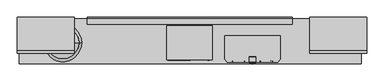
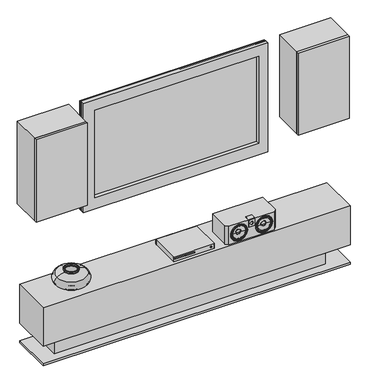
"""IFC4 building model written with IfcOpenShell, lengths in millimetres: furniture geometry."""

from ifc_helpers import new_model, si_unit, point, frame, frame_2d, origin, place, context, project, spatial, polyline, circle_curve, ellipse_curve, trimmed, segment, composite_curve, outline, extrude, source, transform, mapped, element, save
from ifc_brep_helpers import plane_surface, cylinder_surface, revolved_surface, advanced_brep


def furniture_82e6548d(model_context):
    return source(origin(), model_context, "Body", "SolidModel", [
        advanced_brep(
        [(-639.7449376, -196.5814234, 623.1824519), (-549.7449376, -196.5814234, 623.1824519), (-552.6293304, -196.5814234, 620.2980592), (-636.8605449, -196.5814234, 620.2980592), (-639.7449376, -196.5814234, 624.4168309), (-549.7449376, -196.5814234, 624.4168309), (-642.5429469, -196.5814234, 628.1680622), (-546.9469284, -196.5814234, 628.1680622), (-732.6689597, -196.5814234, 648.0450381), (-456.8209156, -196.5814234, 648.0450381), (-737.117516, -196.5814234, 732.9285485), (-452.3723593, -196.5814234, 732.9285485), (-662.9428076, -196.5814234, 762.897076), (-526.5470677, -196.5814234, 762.897076), (-655.9949338, -196.5814234, 766.1369227), (-533.4949414, -196.5814234, 766.1369227), (-660.6249856, -196.5814234, 773.2665773), (-528.8648897, -196.5814234, 773.2665773), (-660.6249856, -196.5814234, 780.1412568), (-528.8648897, -196.5814234, 780.1412568), (-652.9929948, -196.5814234, 780.1412568), (-536.4968805, -196.5814234, 780.1412568), (-649.5413299, -196.5814234, 775.2117685), (-539.9485454, -196.5814234, 775.2117685), (-651.8181703, -196.5814234, 761.8066565), (-537.671705, -196.5814234, 761.8066565), (-661.7982324, -196.5814234, 757.0072587), (-527.6916429, -196.5814234, 757.0072587), (-733.8494437, -196.5814234, 727.8966798), (-455.6404316, -196.5814234, 727.8966798), (-729.9447637, -196.5814234, 653.3909483), (-459.5451115, -196.5814234, 653.3909483), (-639.3868915, -196.5814234, 634.3217368), (-550.1029838, -196.5814234, 634.3217368), (-632.2712578, -196.5814234, 629.6724919), (-557.2186175, -196.5814234, 629.6724919), (-626.4265689, -196.5814234, 626.2980592), (-563.0633064, -196.5814234, 626.2980592), (-594.7449376, -196.5814234, 626.2980592), (-594.7449376, -196.5814234, 620.2980592)],
        [
            (0, 1, circle_curve(frame((-594.7449376, -196.5814234, 623.1824519), z_axis=(0.0, 0.0, -1.0), x_axis=(1.0, 0.0, 0.0)), 45.0)),
            (1, 2, circle_curve(frame((-552.6293304, -196.5814234, 623.1824519), z_axis=(0.0, 1.0, 0.0), x_axis=(1.0, 0.0, 0.0)), 2.8843927)),
            (2, 3, circle_curve(frame((-594.7449376, -196.5814234, 620.2980592), z_axis=(0.0, 0.0, 1.0), x_axis=(1.0, 0.0, 0.0)), 42.1156073)),
            (3, 0, circle_curve(frame((-636.8605449, -196.5814234, 623.1824519), z_axis=(0.0, 1.0, 0.0), x_axis=(-1.0, 0.0, 0.0)), 2.8843927)),
            (1, 0, circle_curve(frame((-594.7449376, -196.5814234, 623.1824519), z_axis=(0.0, 0.0, -1.0), x_axis=(1.0, 0.0, 0.0)), 45.0)),
            (3, 2, circle_curve(frame((-594.7449376, -196.5814234, 620.2980592), z_axis=(0.0, 0.0, 1.0), x_axis=(1.0, 0.0, 0.0)), 42.1156073)),
            (4, 5, circle_curve(frame((-594.7449376, -196.5814234, 624.4168309), z_axis=(0.0, 0.0, -1.0), x_axis=(1.0, 0.0, 0.0)), 45.0)),
            (5, 1),
            (0, 4),
            (5, 4, circle_curve(frame((-594.7449376, -196.5814234, 624.4168309), z_axis=(0.0, 0.0, -1.0), x_axis=(1.0, 0.0, 0.0)), 45.0)),
            (6, 7, circle_curve(frame((-594.7449376, -196.5814234, 628.1680622), z_axis=(0.0, 0.0, -1.0), x_axis=(1.0, 0.0, 0.0)), 47.7980093)),
            (7, 5, circle_curve(frame((-545.7501654, -196.5814234, 624.3562871), z_axis=(0.0, -1.0, 0.0), x_axis=(1.0, 0.0, 0.0)), 3.995231)),
            (4, 6, circle_curve(frame((-643.7397099, -196.5814234, 624.3562871), z_axis=(0.0, -1.0, 0.0), x_axis=(-1.0, 0.0, 0.0)), 3.995231)),
            (7, 6, circle_curve(frame((-594.7449376, -196.5814234, 628.1680622), z_axis=(0.0, 0.0, -1.0), x_axis=(1.0, 0.0, 0.0)), 47.7980093)),
            (8, 9, circle_curve(frame((-594.7449376, -196.5814234, 648.0450381), z_axis=(0.0, 0.0, -1.0), x_axis=(1.0, 0.0, 0.0)), 137.9240221)),
            (9, 7, circle_curve(frame((-540.1329588, -196.5814234, 811.5350037), z_axis=(0.0, 1.0, 0.0), x_axis=(1.0, 0.0, 0.0)), 183.4935024)),
            (6, 8, circle_curve(frame((-649.3569165, -196.5814234, 811.5350037), z_axis=(0.0, 1.0, 0.0), x_axis=(-1.0, 0.0, 0.0)), 183.4935024)),
            (9, 8, circle_curve(frame((-594.7449376, -196.5814234, 648.0450381), z_axis=(0.0, 0.0, -1.0), x_axis=(1.0, 0.0, 0.0)), 137.9240221)),
            (10, 11, circle_curve(frame((-594.7449376, -196.5814234, 732.9285485), z_axis=(0.0, 0.0, -1.0), x_axis=(1.0, 0.0, 0.0)), 142.3725784)),
            (11, 9, circle_curve(frame((-479.1030741, -196.5814234, 691.7711212), z_axis=(0.0, 1.0, 0.0), x_axis=(1.0, 0.0, 0.0)), 49.0761137)),
            (8, 10, circle_curve(frame((-710.3868012, -196.5814234, 691.7711212), z_axis=(0.0, 1.0, 0.0), x_axis=(-1.0, 0.0, 0.0)), 49.0761137)),
            (11, 10, circle_curve(frame((-594.7449376, -196.5814234, 732.9285485), z_axis=(0.0, 0.0, -1.0), x_axis=(1.0, 0.0, 0.0)), 142.3725784)),
            (12, 13, circle_curve(frame((-594.7449376, -196.5814234, 762.897076), z_axis=(0.0, 0.0, -1.0), x_axis=(1.0, 0.0, 0.0)), 68.19787)),
            (13, 11, circle_curve(frame((-566.5275973, -196.5814234, 557.1631061), z_axis=(0.0, 1.0, 0.0), x_axis=(1.0, 0.0, 0.0)), 209.5827023)),
            (10, 12, circle_curve(frame((-622.962278, -196.5814234, 557.1631061), z_axis=(0.0, 1.0, 0.0), x_axis=(-1.0, 0.0, 0.0)), 209.5827023)),
            (13, 12, circle_curve(frame((-594.7449376, -196.5814234, 762.897076), z_axis=(0.0, 0.0, -1.0), x_axis=(1.0, 0.0, 0.0)), 68.19787)),
            (14, 15, circle_curve(frame((-594.7449376, -196.5814234, 766.1369227), z_axis=(0.0, 0.0, -1.0), x_axis=(1.0, 0.0, 0.0)), 61.2499962)),
            (15, 13, circle_curve(frame((-523.5251563, -196.5814234, 778.447391), z_axis=(0.0, -1.0, 0.0), x_axis=(1.0, 0.0, 0.0)), 15.8412198)),
            (12, 14, circle_curve(frame((-665.964719, -196.5814234, 778.447391), z_axis=(0.0, -1.0, 0.0), x_axis=(-1.0, 0.0, 0.0)), 15.8412198)),
            (15, 14, circle_curve(frame((-594.7449376, -196.5814234, 766.1369227), z_axis=(0.0, 0.0, -1.0), x_axis=(1.0, 0.0, 0.0)), 61.2499962)),
            (16, 17, circle_curve(frame((-594.7449376, -196.5814234, 773.2665773), z_axis=(0.0, 0.0, -1.0), x_axis=(1.0, 0.0, 0.0)), 65.880048)),
            (17, 15, circle_curve(frame((-530.8050666, -196.5814234, 769.4583202), z_axis=(0.0, -1.0, 0.0), x_axis=(1.0, 0.0, 0.0)), 4.2740038)),
            (14, 16, circle_curve(frame((-658.6848087, -196.5814234, 769.4583202), z_axis=(0.0, -1.0, 0.0), x_axis=(-1.0, 0.0, 0.0)), 4.2740038)),
            (17, 16, circle_curve(frame((-594.7449376, -196.5814234, 773.2665773), z_axis=(0.0, 0.0, -1.0), x_axis=(1.0, 0.0, 0.0)), 65.880048)),
            (18, 19, circle_curve(frame((-594.7449376, -196.5814234, 780.1412568), z_axis=(0.0, 0.0, -1.0), x_axis=(1.0, 0.0, 0.0)), 65.880048)),
            (19, 17, circle_curve(frame((-528.8648897, -196.5814234, 776.703917), z_axis=(0.0, 1.0, 0.0), x_axis=(1.0, 0.0, 0.0)), 3.4373398)),
            (16, 18, circle_curve(frame((-660.6249856, -196.5814234, 776.703917), z_axis=(0.0, 1.0, 0.0), x_axis=(-1.0, 0.0, 0.0)), 3.4373398)),
            (19, 18, circle_curve(frame((-594.7449376, -196.5814234, 780.1412568), z_axis=(0.0, 0.0, -1.0), x_axis=(1.0, 0.0, 0.0)), 65.880048)),
            (20, 21, circle_curve(frame((-594.7449376, -196.5814234, 780.1412568), z_axis=(0.0, 0.0, -1.0), x_axis=(1.0, 0.0, 0.0)), 58.2480571)),
            (21, 19),
            (18, 20),
            (21, 20, circle_curve(frame((-594.7449376, -196.5814234, 780.1412568), z_axis=(0.0, 0.0, -1.0), x_axis=(1.0, 0.0, 0.0)), 58.2480571)),
            (22, 23, circle_curve(frame((-594.7449376, -196.5814234, 775.2117685), z_axis=(0.0, 0.0, -1.0), x_axis=(1.0, 0.0, 0.0)), 54.7963923)),
            (23, 21, circle_curve(frame((-536.4968805, -196.5814234, 776.4680717), z_axis=(0.0, 1.0, 0.0), x_axis=(1.0, 0.0, 0.0)), 3.673185)),
            (20, 22, circle_curve(frame((-652.9929948, -196.5814234, 776.4680717), z_axis=(0.0, 1.0, 0.0), x_axis=(-1.0, 0.0, 0.0)), 3.673185)),
            (23, 22, circle_curve(frame((-594.7449376, -196.5814234, 775.2117685), z_axis=(0.0, 0.0, -1.0), x_axis=(1.0, 0.0, 0.0)), 54.7963923)),
            (24, 25, circle_curve(frame((-594.7449376, -196.5814234, 761.8066565), z_axis=(0.0, 0.0, -1.0), x_axis=(1.0, 0.0, 0.0)), 57.0732327)),
            (25, 23, circle_curve(frame((-508.2403508, -196.5814234, 773.7014481), z_axis=(0.0, 1.0, 0.0), x_axis=(1.0, 0.0, 0.0)), 31.7441439)),
            (22, 24, circle_curve(frame((-681.2495245, -196.5814234, 773.7014481), z_axis=(0.0, 1.0, 0.0), x_axis=(-1.0, 0.0, 0.0)), 31.7441439)),
            (25, 24, circle_curve(frame((-594.7449376, -196.5814234, 761.8066565), z_axis=(0.0, 0.0, -1.0), x_axis=(1.0, 0.0, 0.0)), 57.0732327)),
            (26, 27, circle_curve(frame((-594.7449376, -196.5814234, 757.0072587), z_axis=(0.0, 0.0, -1.0), x_axis=(1.0, 0.0, 0.0)), 67.0532947)),
            (27, 25, circle_curve(frame((-523.5251563, -196.5814234, 778.447391), z_axis=(0.0, 1.0, 0.0), x_axis=(1.0, 0.0, 0.0)), 21.8412198)),
            (24, 26, circle_curve(frame((-665.964719, -196.5814234, 778.447391), z_axis=(0.0, 1.0, 0.0), x_axis=(-1.0, 0.0, 0.0)), 21.8412198)),
            (27, 26, circle_curve(frame((-594.7449376, -196.5814234, 757.0072587), z_axis=(0.0, 0.0, -1.0), x_axis=(1.0, 0.0, 0.0)), 67.0532947)),
            (28, 29, circle_curve(frame((-594.7449376, -196.5814234, 727.8966798), z_axis=(0.0, 0.0, -1.0), x_axis=(1.0, 0.0, 0.0)), 139.104506)),
            (29, 27, circle_curve(frame((-566.5275973, -196.5814234, 557.1631061), z_axis=(0.0, -1.0, 0.0), x_axis=(1.0, 0.0, 0.0)), 203.5827023)),
            (26, 28, circle_curve(frame((-622.962278, -196.5814234, 557.1631061), z_axis=(0.0, -1.0, 0.0), x_axis=(-1.0, 0.0, 0.0)), 203.5827023)),
            (29, 28, circle_curve(frame((-594.7449376, -196.5814234, 727.8966798), z_axis=(0.0, 0.0, -1.0), x_axis=(1.0, 0.0, 0.0)), 139.104506)),
            (30, 31, circle_curve(frame((-594.7449376, -196.5814234, 653.3909483), z_axis=(0.0, 0.0, -1.0), x_axis=(1.0, 0.0, 0.0)), 135.1998261)),
            (31, 29, circle_curve(frame((-479.1030741, -196.5814234, 691.7711212), z_axis=(0.0, -1.0, 0.0), x_axis=(1.0, 0.0, 0.0)), 43.0761137)),
            (28, 30, circle_curve(frame((-710.3868012, -196.5814234, 691.7711212), z_axis=(0.0, -1.0, 0.0), x_axis=(-1.0, 0.0, 0.0)), 43.0761137)),
            (31, 30, circle_curve(frame((-594.7449376, -196.5814234, 653.3909483), z_axis=(0.0, 0.0, -1.0), x_axis=(1.0, 0.0, 0.0)), 135.1998261)),
            (32, 33, circle_curve(frame((-594.7449376, -196.5814234, 634.3217368), z_axis=(0.0, 0.0, -1.0), x_axis=(1.0, 0.0, 0.0)), 44.6419538)),
            (33, 31, circle_curve(frame((-540.1329588, -196.5814234, 811.5350037), z_axis=(0.0, -1.0, 0.0), x_axis=(1.0, 0.0, 0.0)), 177.4935024)),
            (30, 32, circle_curve(frame((-649.3569165, -196.5814234, 811.5350037), z_axis=(0.0, -1.0, 0.0), x_axis=(-1.0, 0.0, 0.0)), 177.4935024)),
            (33, 32, circle_curve(frame((-594.7449376, -196.5814234, 634.3217368), z_axis=(0.0, 0.0, -1.0), x_axis=(1.0, 0.0, 0.0)), 44.6419538)),
            (34, 35, circle_curve(frame((-594.7449376, -196.5814234, 629.6724919), z_axis=(0.0, 0.0, -1.0), x_axis=(1.0, 0.0, 0.0)), 37.5263202)),
            (35, 33, circle_curve(frame((-549.3684369, -196.5814234, 625.4276845), z_axis=(0.0, 1.0, 0.0), x_axis=(1.0, 0.0, 0.0)), 8.9243333)),
            (32, 34, circle_curve(frame((-640.1214384, -196.5814234, 625.4276845), z_axis=(0.0, 1.0, 0.0), x_axis=(-1.0, 0.0, 0.0)), 8.9243333)),
            (35, 34, circle_curve(frame((-594.7449376, -196.5814234, 629.6724919), z_axis=(0.0, 0.0, -1.0), x_axis=(1.0, 0.0, 0.0)), 37.5263202)),
            (36, 37, circle_curve(frame((-594.7449376, -196.5814234, 626.2980592), z_axis=(0.0, 0.0, -1.0), x_axis=(1.0, 0.0, 0.0)), 31.6816313)),
            (37, 35, circle_curve(frame((-563.1842649, -196.5814234, 633.2564309), z_axis=(0.0, -1.0, 0.0), x_axis=(1.0, 0.0, 0.0)), 6.9594229)),
            (34, 36, circle_curve(frame((-626.3056104, -196.5814234, 633.2564309), z_axis=(0.0, -1.0, 0.0), x_axis=(-1.0, 0.0, 0.0)), 6.9594229)),
            (37, 36, circle_curve(frame((-594.7449376, -196.5814234, 626.2980592), z_axis=(0.0, 0.0, -1.0), x_axis=(1.0, 0.0, 0.0)), 31.6816313)),
            (38, 37),
            (36, 38),
            (2, 39),
            (39, 3),
        ],
        [
            revolved_surface(trimmed(ellipse_curve(frame((-552.6293304, -196.5814234, 623.1824519), z_axis=(0.0, -1.0, 0.0), x_axis=(1.0, 0.0, 0.0)), 2.8843927, 2.8843927), [point((-552.6293304, -196.5814234, 620.2980592))], [point((-549.7449376, -196.5814234, 623.1824519))], True, "CARTESIAN"), (-594.7449376, -196.5814234, 800.1412568), (0.0, 0.0, 1.0)),
            cylinder_surface(frame((-594.7449376, -196.5814234, 800.1412568), z_axis=(0.0, 0.0, 1.0), x_axis=(1.0, 0.0, 0.0)), 45.0),
            revolved_surface(trimmed(ellipse_curve(frame((-545.7501654, -196.5814234, 624.3562871), z_axis=(0.0, 1.0, 0.0), x_axis=(1.0, 0.0, 0.0)), 3.995231, 3.995231), [point((-549.7449376, -196.5814234, 624.4168309))], [point((-546.9469284, -196.5814234, 628.1680622))], True, "CARTESIAN"), (-594.7449376, -196.5814234, 800.1412568), (0.0, 0.0, 1.0)),
            revolved_surface(trimmed(ellipse_curve(frame((-540.1329588, -196.5814234, 811.5350037), z_axis=(0.0, -1.0, 0.0), x_axis=(1.0, 0.0, 0.0)), 183.4935024, 183.4935024), [point((-546.9469284, -196.5814234, 628.1680622))], [point((-456.8209156, -196.5814234, 648.0450381))], True, "CARTESIAN"), (-594.7449376, -196.5814234, 800.1412568), (0.0, 0.0, 1.0)),
            revolved_surface(trimmed(ellipse_curve(frame((-479.1030741, -196.5814234, 691.7711212), z_axis=(0.0, -1.0, 0.0), x_axis=(1.0, 0.0, 0.0)), 49.0761137, 49.0761137), [point((-456.8209156, -196.5814234, 648.0450381))], [point((-452.3723593, -196.5814234, 732.9285485))], True, "CARTESIAN"), (-594.7449376, -196.5814234, 800.1412568), (0.0, 0.0, 1.0)),
            revolved_surface(trimmed(ellipse_curve(frame((-566.5275973, -196.5814234, 557.1631061), z_axis=(0.0, -1.0, 0.0), x_axis=(1.0, 0.0, 0.0)), 209.5827023, 209.5827023), [point((-452.3723593, -196.5814234, 732.9285485))], [point((-526.5470677, -196.5814234, 762.897076))], True, "CARTESIAN"), (-594.7449376, -196.5814234, 800.1412568), (0.0, 0.0, 1.0)),
            revolved_surface(trimmed(ellipse_curve(frame((-523.5251563, -196.5814234, 778.447391), z_axis=(0.0, 1.0, 0.0), x_axis=(1.0, 0.0, 0.0)), 15.8412198, 15.8412198), [point((-526.5470677, -196.5814234, 762.897076))], [point((-533.4949414, -196.5814234, 766.1369227))], True, "CARTESIAN"), (-594.7449376, -196.5814234, 800.1412568), (0.0, 0.0, 1.0)),
            revolved_surface(trimmed(ellipse_curve(frame((-530.8050666, -196.5814234, 769.4583202), z_axis=(0.0, 1.0, 0.0), x_axis=(1.0, 0.0, 0.0)), 4.2740038, 4.2740038), [point((-533.4949414, -196.5814234, 766.1369227))], [point((-528.8648897, -196.5814234, 773.2665773))], True, "CARTESIAN"), (-594.7449376, -196.5814234, 800.1412568), (0.0, 0.0, 1.0)),
            revolved_surface(trimmed(ellipse_curve(frame((-528.8648897, -196.5814234, 776.703917), z_axis=(0.0, -1.0, 0.0), x_axis=(1.0, 0.0, 0.0)), 3.4373398, 3.4373398), [point((-528.8648897, -196.5814234, 773.2665773))], [point((-528.8648897, -196.5814234, 780.1412568))], True, "CARTESIAN"), (-594.7449376, -196.5814234, 800.1412568), (0.0, 0.0, 1.0)),
            plane_surface(frame((-594.7449376, -196.5814234, 780.1412568), z_axis=(0.0, 0.0, 1.0), x_axis=(1.0, 0.0, 0.0))),
            revolved_surface(trimmed(ellipse_curve(frame((-536.4968805, -196.5814234, 776.4680717), z_axis=(0.0, -1.0, 0.0), x_axis=(1.0, 0.0, 0.0)), 3.673185, 3.673185), [point((-536.4968805, -196.5814234, 780.1412568))], [point((-539.9485454, -196.5814234, 775.2117685))], True, "CARTESIAN"), (-594.7449376, -196.5814234, 800.1412568), (0.0, 0.0, 1.0)),
            revolved_surface(trimmed(ellipse_curve(frame((-508.2403508, -196.5814234, 773.7014481), z_axis=(0.0, -1.0, 0.0), x_axis=(1.0, 0.0, 0.0)), 31.7441439, 31.7441439), [point((-539.9485454, -196.5814234, 775.2117685))], [point((-537.671705, -196.5814234, 761.8066565))], True, "CARTESIAN"), (-594.7449376, -196.5814234, 800.1412568), (0.0, 0.0, 1.0)),
            revolved_surface(trimmed(ellipse_curve(frame((-523.5251563, -196.5814234, 778.447391), z_axis=(0.0, -1.0, 0.0), x_axis=(1.0, 0.0, 0.0)), 21.8412198, 21.8412198), [point((-537.671705, -196.5814234, 761.8066565))], [point((-527.6916429, -196.5814234, 757.0072587))], True, "CARTESIAN"), (-594.7449376, -196.5814234, 800.1412568), (0.0, 0.0, 1.0)),
            revolved_surface(trimmed(ellipse_curve(frame((-566.5275973, -196.5814234, 557.1631061), z_axis=(0.0, 1.0, 0.0), x_axis=(1.0, 0.0, 0.0)), 203.5827023, 203.5827023), [point((-527.6916429, -196.5814234, 757.0072587))], [point((-455.6404316, -196.5814234, 727.8966798))], True, "CARTESIAN"), (-594.7449376, -196.5814234, 800.1412568), (0.0, 0.0, 1.0)),
            revolved_surface(trimmed(ellipse_curve(frame((-479.1030741, -196.5814234, 691.7711212), z_axis=(0.0, 1.0, 0.0), x_axis=(1.0, 0.0, 0.0)), 43.0761137, 43.0761137), [point((-455.6404316, -196.5814234, 727.8966798))], [point((-459.5451115, -196.5814234, 653.3909483))], True, "CARTESIAN"), (-594.7449376, -196.5814234, 800.1412568), (0.0, 0.0, 1.0)),
            revolved_surface(trimmed(ellipse_curve(frame((-540.1329588, -196.5814234, 811.5350037), z_axis=(0.0, 1.0, 0.0), x_axis=(1.0, 0.0, 0.0)), 177.4935024, 177.4935024), [point((-459.5451115, -196.5814234, 653.3909483))], [point((-550.1029838, -196.5814234, 634.3217368))], True, "CARTESIAN"), (-594.7449376, -196.5814234, 800.1412568), (0.0, 0.0, 1.0)),
            revolved_surface(trimmed(ellipse_curve(frame((-549.3684369, -196.5814234, 625.4276845), z_axis=(0.0, -1.0, 0.0), x_axis=(1.0, 0.0, 0.0)), 8.9243333, 8.9243333), [point((-550.1029838, -196.5814234, 634.3217368))], [point((-557.2186175, -196.5814234, 629.6724919))], True, "CARTESIAN"), (-594.7449376, -196.5814234, 800.1412568), (0.0, 0.0, 1.0)),
            revolved_surface(trimmed(ellipse_curve(frame((-563.1842649, -196.5814234, 633.2564309), z_axis=(0.0, 1.0, 0.0), x_axis=(1.0, 0.0, 0.0)), 6.9594229, 6.9594229), [point((-557.2186175, -196.5814234, 629.6724919))], [point((-563.0633064, -196.5814234, 626.2980592))], True, "CARTESIAN"), (-594.7449376, -196.5814234, 800.1412568), (0.0, 0.0, 1.0)),
            plane_surface(frame((-594.7449376, -196.5814234, 626.2980592), z_axis=(0.0, 0.0, 1.0), x_axis=(1.0, 0.0, 0.0))),
            plane_surface(frame((-594.7449376, -196.5814234, 620.2980592), z_axis=(0.0, 0.0, -1.0), x_axis=(1.0, 0.0, 0.0))),
        ],
        [
            (0, [[1, 2, 3, 4]]),
            (0, [[5, -4, 6, -2]]),
            (1, [[7, 8, -1, 9]]),
            (1, [[10, -9, -5, -8]]),
            (2, [[11, 12, -7, 13]]),
            (2, [[14, -13, -10, -12]]),
            (3, [[15, 16, -11, 17]]),
            (3, [[18, -17, -14, -16]]),
            (4, [[19, 20, -15, 21]]),
            (4, [[22, -21, -18, -20]]),
            (5, [[23, 24, -19, 25]]),
            (5, [[26, -25, -22, -24]]),
            (6, [[27, 28, -23, 29]]),
            (6, [[30, -29, -26, -28]]),
            (7, [[31, 32, -27, 33]]),
            (7, [[34, -33, -30, -32]]),
            (8, [[35, 36, -31, 37]]),
            (8, [[38, -37, -34, -36]]),
            (9, [[39, 40, -35, 41]]),
            (9, [[42, -41, -38, -40]]),
            (10, [[43, 44, -39, 45]]),
            (10, [[46, -45, -42, -44]]),
            (11, [[47, 48, -43, 49]]),
            (11, [[50, -49, -46, -48]]),
            (12, [[51, 52, -47, 53]]),
            (12, [[54, -53, -50, -52]]),
            (13, [[55, 56, -51, 57]]),
            (13, [[58, -57, -54, -56]]),
            (14, [[59, 60, -55, 61]]),
            (14, [[62, -61, -58, -60]]),
            (15, [[63, 64, -59, 65]]),
            (15, [[66, -65, -62, -64]]),
            (16, [[67, 68, -63, 69]]),
            (16, [[70, -69, -66, -68]]),
            (17, [[71, 72, -67, 73]]),
            (17, [[74, -73, -70, -72]]),
            (18, [[75, -71, 76]]),
            (18, [[-76, -74, -75]]),
            (19, [[-3, 77, 78]]),
            (19, [[-6, -78, -77]]),
        ],
    ),
        advanced_brep(
        [(1262.045258, -367.5, 711.570893), (1119.0326349, -367.5, 711.570893), (1120.5389465, -365.9936884, 711.570893), (1260.5389465, -365.9936884, 711.570893), (1272.0516084, -367.5, 711.570893), (1109.0262846, -367.5, 711.570893), (1273.5389465, -366.0126619, 711.570893), (1107.5389465, -366.0126619, 711.570893), (1273.5389465, -365.0, 711.570893), (1107.5389465, -365.0, 711.570893), (1260.5389465, -365.0, 711.570893), (1120.5389465, -365.0, 711.570893)],
        [
            (0, 1, circle_curve(frame((1190.5389465, -367.5, 711.570893), z_axis=(0.0, -1.0, 0.0), x_axis=(-1.0, 0.0, 0.0)), 71.5063116)),
            (1, 2, circle_curve(frame((1119.0326349, -365.9936884, 711.570893), z_axis=(0.0, 0.0, 1.0), x_axis=(1.0, 0.0, 0.0)), 1.5063116)),
            (2, 3, circle_curve(frame((1190.5389465, -365.9936884, 711.570893), z_axis=(0.0, 1.0, 0.0), x_axis=(-1.0, 0.0, 0.0)), 70.0)),
            (3, 0, circle_curve(frame((1262.045258, -365.9936884, 711.570893), z_axis=(0.0, 0.0, 1.0), x_axis=(-1.0, 0.0, 0.0)), 1.5063116)),
            (1, 0, circle_curve(frame((1190.5389465, -367.5, 711.570893), z_axis=(0.0, -1.0, 0.0), x_axis=(-1.0, 0.0, 0.0)), 71.5063116)),
            (3, 2, circle_curve(frame((1190.5389465, -365.9936884, 711.570893), z_axis=(0.0, 1.0, 0.0), x_axis=(-1.0, 0.0, 0.0)), 70.0)),
            (4, 5, circle_curve(frame((1190.5389465, -367.5, 711.570893), z_axis=(0.0, -1.0, 0.0), x_axis=(-1.0, 0.0, 0.0)), 81.5126619)),
            (5, 1),
            (0, 4),
            (5, 4, circle_curve(frame((1190.5389465, -367.5, 711.570893), z_axis=(0.0, -1.0, 0.0), x_axis=(-1.0, 0.0, 0.0)), 81.5126619)),
            (6, 7, circle_curve(frame((1190.5389465, -366.0126619, 711.570893), z_axis=(0.0, -1.0, 0.0), x_axis=(-1.0, 0.0, 0.0)), 83.0)),
            (7, 5, circle_curve(frame((1109.0262846, -366.0126619, 711.570893), z_axis=(0.0, 0.0, 1.0), x_axis=(1.0, 0.0, 0.0)), 1.4873381)),
            (4, 6, circle_curve(frame((1272.0516084, -366.0126619, 711.570893), z_axis=(0.0, 0.0, 1.0), x_axis=(-1.0, 0.0, 0.0)), 1.4873381)),
            (7, 6, circle_curve(frame((1190.5389465, -366.0126619, 711.570893), z_axis=(0.0, -1.0, 0.0), x_axis=(-1.0, 0.0, 0.0)), 83.0)),
            (8, 9, circle_curve(frame((1190.5389465, -365.0, 711.570893), z_axis=(0.0, -1.0, 0.0), x_axis=(-1.0, 0.0, 0.0)), 83.0)),
            (9, 7),
            (6, 8),
            (9, 8, circle_curve(frame((1190.5389465, -365.0, 711.570893), z_axis=(0.0, -1.0, 0.0), x_axis=(-1.0, 0.0, 0.0)), 83.0)),
            (10, 11, circle_curve(frame((1190.5389465, -365.0, 711.570893), z_axis=(0.0, -1.0, 0.0), x_axis=(-1.0, 0.0, 0.0)), 70.0)),
            (11, 9),
            (8, 10),
            (11, 10, circle_curve(frame((1190.5389465, -365.0, 711.570893), z_axis=(0.0, -1.0, 0.0), x_axis=(-1.0, 0.0, 0.0)), 70.0)),
            (2, 11),
            (10, 3),
        ],
        [
            revolved_surface(trimmed(ellipse_curve(frame((1119.0326349, -365.9936884, 711.570893), z_axis=(0.0, 0.0, -1.0), x_axis=(1.0, 0.0, 0.0)), 1.5063116, 1.5063116), [point((1120.5389465, -365.9936884, 711.570893))], [point((1119.0326349, -367.5, 711.570893))], True, "CARTESIAN"), (1190.5389465, -2974.0581012, 711.570893), (0.0, 1.0, 0.0)),
            plane_surface(frame((1190.5389465, -367.5, 711.570893), z_axis=(0.0, -1.0, 0.0), x_axis=(-1.0, 0.0, 0.0))),
            revolved_surface(trimmed(ellipse_curve(frame((1109.0262846, -366.0126619, 711.570893), z_axis=(0.0, 0.0, -1.0), x_axis=(1.0, 0.0, 0.0)), 1.4873381, 1.4873381), [point((1109.0262846, -367.5, 711.570893))], [point((1107.5389465, -366.0126619, 711.570893))], True, "CARTESIAN"), (1190.5389465, -2974.0581012, 711.570893), (0.0, 1.0, 0.0)),
            cylinder_surface(frame((1190.5389465, -2974.0581012, 711.570893), z_axis=(0.0, 1.0, 0.0), x_axis=(-1.0, 0.0, 0.0)), 83.0),
            plane_surface(frame((1190.5389465, -365.0, 711.570893), z_axis=(0.0, 1.0, 0.0), x_axis=(-1.0, 0.0, 0.0))),
            revolved_surface(polyline([(1120.5389465, -365.0, 711.570893), (1120.5389465, -365.9936883999999, 711.570893)]), (1190.5389465, -2974.0581012, 711.570893), (0.0, 1.0, 0.0)),
        ],
        [
            (0, [[1, 2, 3, 4]]),
            (0, [[5, -4, 6, -2]]),
            (1, [[7, 8, -1, 9]]),
            (1, [[10, -9, -5, -8]]),
            (2, [[11, 12, -7, 13]]),
            (2, [[14, -13, -10, -12]]),
            (3, [[15, 16, -11, 17]]),
            (3, [[18, -17, -14, -16]]),
            (4, [[19, 20, -15, 21]]),
            (4, [[22, -21, -18, -20]]),
            (5, [[-3, 23, -19, 24]]),
            (5, [[-6, -24, -22, -23]]),
        ],
    ),
        advanced_brep(
        [(1190.5389465, -339.519831, 711.570893), (1120.5389465, -339.519831, 711.570893), (1260.5389465, -339.519831, 711.570893), (1210.5389465, -352.7244931, 711.570893), (1170.5389465, -352.7244931, 711.570893), (1190.5389465, -360.9291552, 711.570893), (1215.5389465, -352.7244931, 711.570893), (1165.5389465, -352.7244931, 711.570893), (1252.8404834, -363.2734987, 711.570893), (1128.2374096, -363.2734987, 711.570893), (1257.5389465, -364.9835994, 711.570893), (1123.5389465, -364.9835994, 711.570893), (1260.5389465, -364.9835994, 711.570893), (1120.5389465, -364.9835994, 711.570893)],
        [
            (0, 1),
            (1, 2, circle_curve(frame((1190.5389465, -339.519831, 711.570893), z_axis=(0.0, 1.0, 0.0), x_axis=(-1.0, 0.0, 0.0)), 70.0)),
            (2, 0),
            (2, 1, circle_curve(frame((1190.5389465, -339.519831, 711.570893), z_axis=(0.0, 1.0, 0.0), x_axis=(-1.0, 0.0, 0.0)), 70.0)),
            (3, 4, circle_curve(frame((1190.5389465, -352.7244931, 711.570893), z_axis=(0.0, -1.0, 0.0), x_axis=(-1.0, 0.0, 0.0)), 20.0)),
            (4, 5, circle_curve(frame((1190.5389465, -332.4504394, 711.570893), z_axis=(0.0, 0.0, 1.0), x_axis=(1.0, 0.0, 0.0)), 28.4787158)),
            (5, 3, circle_curve(frame((1190.5389465, -332.4504394, 711.570893), z_axis=(0.0, 0.0, 1.0), x_axis=(-1.0, 0.0, 0.0)), 28.4787158)),
            (4, 3, circle_curve(frame((1190.5389465, -352.7244931, 711.570893), z_axis=(0.0, -1.0, 0.0), x_axis=(-1.0, 0.0, 0.0)), 20.0)),
            (6, 7, circle_curve(frame((1190.5389465, -352.7244931, 711.570893), z_axis=(0.0, -1.0, 0.0), x_axis=(-1.0, 0.0, 0.0)), 25.0)),
            (7, 4, circle_curve(frame((1168.0389465, -355.2587498, 711.570893), z_axis=(0.0, 0.0, -1.0), x_axis=(1.0, 0.0, 0.0)), 3.5598395)),
            (3, 6, circle_curve(frame((1213.0389465, -355.2587498, 711.570893), z_axis=(0.0, 0.0, -1.0), x_axis=(-1.0, 0.0, 0.0)), 3.5598395)),
            (7, 6, circle_curve(frame((1190.5389465, -352.7244931, 711.570893), z_axis=(0.0, -1.0, 0.0), x_axis=(-1.0, 0.0, 0.0)), 25.0)),
            (8, 9, circle_curve(frame((1190.5389465, -363.2734987, 711.570893), z_axis=(0.0, -1.0, 0.0), x_axis=(-1.0, 0.0, 0.0)), 62.3015369)),
            (9, 7, circle_curve(frame((1108.7972546, -223.3085768, 711.570893), z_axis=(0.0, 0.0, 1.0), x_axis=(1.0, 0.0, 0.0)), 141.3085241)),
            (6, 8, circle_curve(frame((1272.2806383, -223.3085768, 711.570893), z_axis=(0.0, 0.0, 1.0), x_axis=(-1.0, 0.0, 0.0)), 141.3085241)),
            (9, 8, circle_curve(frame((1190.5389465, -363.2734987, 711.570893), z_axis=(0.0, -1.0, 0.0), x_axis=(-1.0, 0.0, 0.0)), 62.3015369)),
            (10, 11, circle_curve(frame((1190.5389465, -364.9835994, 711.570893), z_axis=(0.0, -1.0, 0.0), x_axis=(-1.0, 0.0, 0.0)), 67.0)),
            (11, 9, circle_curve(frame((1126.5872433, -366.049215, 711.570893), z_axis=(0.0, 0.0, -1.0), x_axis=(1.0, 0.0, 0.0)), 3.2291872)),
            (8, 10, circle_curve(frame((1254.4906497, -366.049215, 711.570893), z_axis=(0.0, 0.0, -1.0), x_axis=(-1.0, 0.0, 0.0)), 3.2291872)),
            (11, 10, circle_curve(frame((1190.5389465, -364.9835994, 711.570893), z_axis=(0.0, -1.0, 0.0), x_axis=(-1.0, 0.0, 0.0)), 67.0)),
            (12, 13, circle_curve(frame((1190.5389465, -364.9835994, 711.570893), z_axis=(0.0, -1.0, 0.0), x_axis=(-1.0, 0.0, 0.0)), 70.0)),
            (13, 11),
            (10, 12),
            (13, 12, circle_curve(frame((1190.5389465, -364.9835994, 711.570893), z_axis=(0.0, -1.0, 0.0), x_axis=(-1.0, 0.0, 0.0)), 70.0)),
            (1, 13),
            (12, 2),
        ],
        [
            plane_surface(frame((1190.5389465, -339.519831, 711.570893), z_axis=(0.0, 1.0, 0.0), x_axis=(-1.0, 0.0, 0.0))),
            revolved_surface(trimmed(ellipse_curve(frame((1190.5389465, -332.4504394, 711.570893), z_axis=(0.0, 0.0, -1.0), x_axis=(1.0, 0.0, 0.0)), 28.4787158, 28.4787158), [point((1190.5389465, -360.9291552, 711.570893))], [point((1170.5389465, -352.7244931, 711.570893))], True, "CARTESIAN"), (1190.5389465, -360.9291552, 711.570893), (0.0, 1.0, 0.0)),
            revolved_surface(trimmed(ellipse_curve(frame((1168.0389465, -355.2587498, 711.570893), z_axis=(0.0, 0.0, 1.0), x_axis=(1.0, 0.0, 0.0)), 3.5598395, 3.5598395), [point((1170.5389465, -352.7244931, 711.570893))], [point((1165.5389465, -352.7244931, 711.570893))], True, "CARTESIAN"), (1190.5389465, -360.9291552, 711.570893), (0.0, 1.0, 0.0)),
            revolved_surface(trimmed(ellipse_curve(frame((1108.7972546, -223.3085768, 711.570893), z_axis=(0.0, 0.0, -1.0), x_axis=(1.0, 0.0, 0.0)), 141.3085241, 141.3085241), [point((1165.5389465, -352.7244931, 711.570893))], [point((1128.2374096, -363.2734987, 711.570893))], True, "CARTESIAN"), (1190.5389465, -360.9291552, 711.570893), (0.0, 1.0, 0.0)),
            revolved_surface(trimmed(ellipse_curve(frame((1126.5872433, -366.049215, 711.570893), z_axis=(0.0, 0.0, 1.0), x_axis=(1.0, 0.0, 0.0)), 3.2291872, 3.2291872), [point((1128.2374096, -363.2734987, 711.570893))], [point((1123.5389465, -364.9835994, 711.570893))], True, "CARTESIAN"), (1190.5389465, -360.9291552, 711.570893), (0.0, 1.0, 0.0)),
            plane_surface(frame((1190.5389465, -364.9835994, 711.570893), z_axis=(0.0, -1.0, 0.0), x_axis=(-1.0, 0.0, 0.0))),
            cylinder_surface(frame((1190.5389465, -360.9291552, 711.570893), z_axis=(0.0, 1.0, 0.0), x_axis=(-1.0, 0.0, 0.0)), 70.0),
        ],
        [
            (0, [[1, 2, 3]]),
            (0, [[-3, 4, -1]]),
            (1, [[5, 6, 7]]),
            (1, [[8, -7, -6]]),
            (2, [[9, 10, -5, 11]]),
            (2, [[12, -11, -8, -10]]),
            (3, [[13, 14, -9, 15]]),
            (3, [[16, -15, -12, -14]]),
            (4, [[17, 18, -13, 19]]),
            (4, [[20, -19, -16, -18]]),
            (5, [[21, 22, -17, 23]]),
            (5, [[24, -23, -20, -22]]),
            (6, [[-2, 25, -21, 26]]),
            (6, [[-4, -26, -24, -25]]),
        ],
    ),
        advanced_brep(
        [(1068.0389465, -385.0, 770.320893), (1068.0389465, -370.0, 785.320893), (1068.0389465, -370.0, 755.320893), (1068.0389465, -370.0, 770.320893)],
        [
            (0, 1),
            (1, 2, circle_curve(frame((1068.0389465, -370.0, 770.320893), z_axis=(0.0, -1.0, 0.0), x_axis=(0.0, 0.0, 1.0)), 15.0)),
            (2, 0),
            (2, 1, circle_curve(frame((1068.0389465, -370.0, 770.320893), z_axis=(0.0, -1.0, 0.0), x_axis=(0.0, 0.0, 1.0)), 15.0)),
            (1, 3),
            (3, 2),
        ],
        [
            revolved_surface(polyline([(1068.0389465, -370.0, 785.320893), (1068.0389465, -385.0, 770.320893)]), (1068.0389465, -400.0, 770.320893), (0.0, -1.0, 0.0)),
            plane_surface(frame((1068.0389465, -370.0, 770.320893), z_axis=(0.0, 1.0, 0.0), x_axis=(0.0, 0.0, 1.0))),
        ],
        [
            (0, [[1, 2, 3]]),
            (0, [[-3, 4, -1]]),
            (1, [[-2, 5, 6]]),
            (1, [[-4, -6, -5]]),
        ],
    ),
        extrude(outline(composite_curve([segment(polyline([(-315.0, 806.570893), (-365.0, 806.570893), (-365.0, 731.570893), (-370.0, 734.070893), (-370.0, 806.570893)]), True, "CONTINUOUS"), segment(trimmed(circle_curve(frame_2d((-365.0, 806.570893)), 5.0), [point((-370.0, 806.570893))], [point((-365.0, 811.570893))], False, "CARTESIAN"), True, "CONTINUOUS"), segment(polyline([(-365.0, 811.570893), (-317.5, 811.570893), (-315.0, 806.570893)]), True, "CONTINUOUS")], self_intersect=False)), frame((1038.0389465, 0.0, 0.0), z_axis=(1.0, 0.0, 0.0), x_axis=(0.0, 1.0, 0.0)), (0.0, 0.0, 1.0), 60.0),
        advanced_brep(
        [(1017.045258, -367.5, 711.570893), (874.0326349, -367.5, 711.570893), (875.5389465, -365.9936884, 711.570893), (1015.5389465, -365.9936884, 711.570893), (1027.0516084, -367.5, 711.570893), (864.0262846, -367.5, 711.570893), (1028.5389465, -366.0126619, 711.570893), (862.5389465, -366.0126619, 711.570893), (1028.5389465, -365.0, 711.570893), (862.5389465, -365.0, 711.570893), (1015.5389465, -365.0, 711.570893), (875.5389465, -365.0, 711.570893)],
        [
            (0, 1, circle_curve(frame((945.5389465, -367.5, 711.570893), z_axis=(0.0, -1.0, 0.0), x_axis=(-1.0, 0.0, 0.0)), 71.5063116)),
            (1, 2, circle_curve(frame((874.0326349, -365.9936884, 711.570893), z_axis=(0.0, 0.0, 1.0), x_axis=(1.0, 0.0, 0.0)), 1.5063116)),
            (2, 3, circle_curve(frame((945.5389465, -365.9936884, 711.570893), z_axis=(0.0, 1.0, 0.0), x_axis=(-1.0, 0.0, 0.0)), 70.0)),
            (3, 0, circle_curve(frame((1017.045258, -365.9936884, 711.570893), z_axis=(0.0, 0.0, 1.0), x_axis=(-1.0, 0.0, 0.0)), 1.5063116)),
            (1, 0, circle_curve(frame((945.5389465, -367.5, 711.570893), z_axis=(0.0, -1.0, 0.0), x_axis=(-1.0, 0.0, 0.0)), 71.5063116)),
            (3, 2, circle_curve(frame((945.5389465, -365.9936884, 711.570893), z_axis=(0.0, 1.0, 0.0), x_axis=(-1.0, 0.0, 0.0)), 70.0)),
            (4, 5, circle_curve(frame((945.5389465, -367.5, 711.570893), z_axis=(0.0, -1.0, 0.0), x_axis=(-1.0, 0.0, 0.0)), 81.5126619)),
            (5, 1),
            (0, 4),
            (5, 4, circle_curve(frame((945.5389465, -367.5, 711.570893), z_axis=(0.0, -1.0, 0.0), x_axis=(-1.0, 0.0, 0.0)), 81.5126619)),
            (6, 7, circle_curve(frame((945.5389465, -366.0126619, 711.570893), z_axis=(0.0, -1.0, 0.0), x_axis=(-1.0, 0.0, 0.0)), 83.0)),
            (7, 5, circle_curve(frame((864.0262846, -366.0126619, 711.570893), z_axis=(0.0, 0.0, 1.0), x_axis=(1.0, 0.0, 0.0)), 1.4873381)),
            (4, 6, circle_curve(frame((1027.0516084, -366.0126619, 711.570893), z_axis=(0.0, 0.0, 1.0), x_axis=(-1.0, 0.0, 0.0)), 1.4873381)),
            (7, 6, circle_curve(frame((945.5389465, -366.0126619, 711.570893), z_axis=(0.0, -1.0, 0.0), x_axis=(-1.0, 0.0, 0.0)), 83.0)),
            (8, 9, circle_curve(frame((945.5389465, -365.0, 711.570893), z_axis=(0.0, -1.0, 0.0), x_axis=(-1.0, 0.0, 0.0)), 83.0)),
            (9, 7),
            (6, 8),
            (9, 8, circle_curve(frame((945.5389465, -365.0, 711.570893), z_axis=(0.0, -1.0, 0.0), x_axis=(-1.0, 0.0, 0.0)), 83.0)),
            (10, 11, circle_curve(frame((945.5389465, -365.0, 711.570893), z_axis=(0.0, -1.0, 0.0), x_axis=(-1.0, 0.0, 0.0)), 70.0)),
            (11, 9),
            (8, 10),
            (11, 10, circle_curve(frame((945.5389465, -365.0, 711.570893), z_axis=(0.0, -1.0, 0.0), x_axis=(-1.0, 0.0, 0.0)), 70.0)),
            (2, 11),
            (10, 3),
        ],
        [
            revolved_surface(trimmed(ellipse_curve(frame((874.0326349, -365.9936884, 711.570893), z_axis=(0.0, 0.0, -1.0), x_axis=(1.0, 0.0, 0.0)), 1.5063116, 1.5063116), [point((875.5389465, -365.9936884, 711.570893))], [point((874.0326349, -367.5, 711.570893))], True, "CARTESIAN"), (945.5389465, -2974.0581012, 711.570893), (0.0, 1.0, 0.0)),
            plane_surface(frame((945.5389465, -367.5, 711.570893), z_axis=(0.0, -1.0, 0.0), x_axis=(-1.0, 0.0, 0.0))),
            revolved_surface(trimmed(ellipse_curve(frame((864.0262846, -366.0126619, 711.570893), z_axis=(0.0, 0.0, -1.0), x_axis=(1.0, 0.0, 0.0)), 1.4873381, 1.4873381), [point((864.0262846, -367.5, 711.570893))], [point((862.5389465, -366.0126619, 711.570893))], True, "CARTESIAN"), (945.5389465, -2974.0581012, 711.570893), (0.0, 1.0, 0.0)),
            cylinder_surface(frame((945.5389465, -2974.0581012, 711.570893), z_axis=(0.0, 1.0, 0.0), x_axis=(-1.0, 0.0, 0.0)), 83.0),
            plane_surface(frame((945.5389465, -365.0, 711.570893), z_axis=(0.0, 1.0, 0.0), x_axis=(-1.0, 0.0, 0.0))),
            revolved_surface(polyline([(875.5389465, -365.0, 711.570893), (875.5389465, -365.9936883999999, 711.570893)]), (945.5389465, -2974.0581012, 711.570893), (0.0, 1.0, 0.0)),
        ],
        [
            (0, [[1, 2, 3, 4]]),
            (0, [[5, -4, 6, -2]]),
            (1, [[7, 8, -1, 9]]),
            (1, [[10, -9, -5, -8]]),
            (2, [[11, 12, -7, 13]]),
            (2, [[14, -13, -10, -12]]),
            (3, [[15, 16, -11, 17]]),
            (3, [[18, -17, -14, -16]]),
            (4, [[19, 20, -15, 21]]),
            (4, [[22, -21, -18, -20]]),
            (5, [[-3, 23, -19, 24]]),
            (5, [[-6, -24, -22, -23]]),
        ],
    ),
        advanced_brep(
        [(945.5389465, -339.519831, 711.570893), (875.5389465, -339.519831, 711.570893), (1015.5389465, -339.519831, 711.570893), (965.5389465, -352.7244931, 711.570893), (925.5389465, -352.7244931, 711.570893), (945.5389465, -360.9291552, 711.570893), (970.5389465, -352.7244931, 711.570893), (920.5389465, -352.7244931, 711.570893), (1007.8404834, -363.2734987, 711.570893), (883.2374096, -363.2734987, 711.570893), (1012.5389465, -364.9835994, 711.570893), (878.5389465, -364.9835994, 711.570893), (1015.5389465, -364.9835994, 711.570893), (875.5389465, -364.9835994, 711.570893)],
        [
            (0, 1),
            (1, 2, circle_curve(frame((945.5389465, -339.519831, 711.570893), z_axis=(0.0, 1.0, 0.0), x_axis=(-1.0, 0.0, 0.0)), 70.0)),
            (2, 0),
            (2, 1, circle_curve(frame((945.5389465, -339.519831, 711.570893), z_axis=(0.0, 1.0, 0.0), x_axis=(-1.0, 0.0, 0.0)), 70.0)),
            (3, 4, circle_curve(frame((945.5389465, -352.7244931, 711.570893), z_axis=(0.0, -1.0, 0.0), x_axis=(-1.0, 0.0, 0.0)), 20.0)),
            (4, 5, circle_curve(frame((945.5389465, -332.4504394, 711.570893), z_axis=(0.0, 0.0, 1.0), x_axis=(1.0, 0.0, 0.0)), 28.4787158)),
            (5, 3, circle_curve(frame((945.5389465, -332.4504394, 711.570893), z_axis=(0.0, 0.0, 1.0), x_axis=(-1.0, 0.0, 0.0)), 28.4787158)),
            (4, 3, circle_curve(frame((945.5389465, -352.7244931, 711.570893), z_axis=(0.0, -1.0, 0.0), x_axis=(-1.0, 0.0, 0.0)), 20.0)),
            (6, 7, circle_curve(frame((945.5389465, -352.7244931, 711.570893), z_axis=(0.0, -1.0, 0.0), x_axis=(-1.0, 0.0, 0.0)), 25.0)),
            (7, 4, circle_curve(frame((923.0389465, -355.2587498, 711.570893), z_axis=(0.0, 0.0, -1.0), x_axis=(1.0, 0.0, 0.0)), 3.5598395)),
            (3, 6, circle_curve(frame((968.0389465, -355.2587498, 711.570893), z_axis=(0.0, 0.0, -1.0), x_axis=(-1.0, 0.0, 0.0)), 3.5598395)),
            (7, 6, circle_curve(frame((945.5389465, -352.7244931, 711.570893), z_axis=(0.0, -1.0, 0.0), x_axis=(-1.0, 0.0, 0.0)), 25.0)),
            (8, 9, circle_curve(frame((945.5389465, -363.2734987, 711.570893), z_axis=(0.0, -1.0, 0.0), x_axis=(-1.0, 0.0, 0.0)), 62.3015369)),
            (9, 7, circle_curve(frame((863.7972546, -223.3085768, 711.570893), z_axis=(0.0, 0.0, 1.0), x_axis=(1.0, 0.0, 0.0)), 141.3085241)),
            (6, 8, circle_curve(frame((1027.2806383, -223.3085768, 711.570893), z_axis=(0.0, 0.0, 1.0), x_axis=(-1.0, 0.0, 0.0)), 141.3085241)),
            (9, 8, circle_curve(frame((945.5389465, -363.2734987, 711.570893), z_axis=(0.0, -1.0, 0.0), x_axis=(-1.0, 0.0, 0.0)), 62.3015369)),
            (10, 11, circle_curve(frame((945.5389465, -364.9835994, 711.570893), z_axis=(0.0, -1.0, 0.0), x_axis=(-1.0, 0.0, 0.0)), 67.0)),
            (11, 9, circle_curve(frame((881.5872433, -366.049215, 711.570893), z_axis=(0.0, 0.0, -1.0), x_axis=(1.0, 0.0, 0.0)), 3.2291872)),
            (8, 10, circle_curve(frame((1009.4906497, -366.049215, 711.570893), z_axis=(0.0, 0.0, -1.0), x_axis=(-1.0, 0.0, 0.0)), 3.2291872)),
            (11, 10, circle_curve(frame((945.5389465, -364.9835994, 711.570893), z_axis=(0.0, -1.0, 0.0), x_axis=(-1.0, 0.0, 0.0)), 67.0)),
            (12, 13, circle_curve(frame((945.5389465, -364.9835994, 711.570893), z_axis=(0.0, -1.0, 0.0), x_axis=(-1.0, 0.0, 0.0)), 70.0)),
            (13, 11),
            (10, 12),
            (13, 12, circle_curve(frame((945.5389465, -364.9835994, 711.570893), z_axis=(0.0, -1.0, 0.0), x_axis=(-1.0, 0.0, 0.0)), 70.0)),
            (1, 13),
            (12, 2),
        ],
        [
            plane_surface(frame((945.5389465, -339.519831, 711.570893), z_axis=(0.0, 1.0, 0.0), x_axis=(-1.0, 0.0, 0.0))),
            revolved_surface(trimmed(ellipse_curve(frame((945.5389465, -332.4504394, 711.570893), z_axis=(0.0, 0.0, -1.0), x_axis=(1.0, 0.0, 0.0)), 28.4787158, 28.4787158), [point((945.5389465, -360.9291552, 711.570893))], [point((925.5389465, -352.7244931, 711.570893))], True, "CARTESIAN"), (945.5389465, -360.9291552, 711.570893), (0.0, 1.0, 0.0)),
            revolved_surface(trimmed(ellipse_curve(frame((923.0389465, -355.2587498, 711.570893), z_axis=(0.0, 0.0, 1.0), x_axis=(1.0, 0.0, 0.0)), 3.5598395, 3.5598395), [point((925.5389465, -352.7244931, 711.570893))], [point((920.5389465, -352.7244931, 711.570893))], True, "CARTESIAN"), (945.5389465, -360.9291552, 711.570893), (0.0, 1.0, 0.0)),
            revolved_surface(trimmed(ellipse_curve(frame((863.7972546, -223.3085768, 711.570893), z_axis=(0.0, 0.0, -1.0), x_axis=(1.0, 0.0, 0.0)), 141.3085241, 141.3085241), [point((920.5389465, -352.7244931, 711.570893))], [point((883.2374096, -363.2734987, 711.570893))], True, "CARTESIAN"), (945.5389465, -360.9291552, 711.570893), (0.0, 1.0, 0.0)),
            revolved_surface(trimmed(ellipse_curve(frame((881.5872433, -366.049215, 711.570893), z_axis=(0.0, 0.0, 1.0), x_axis=(1.0, 0.0, 0.0)), 3.2291872, 3.2291872), [point((883.2374096, -363.2734987, 711.570893))], [point((878.5389465, -364.9835994, 711.570893))], True, "CARTESIAN"), (945.5389465, -360.9291552, 711.570893), (0.0, 1.0, 0.0)),
            plane_surface(frame((945.5389465, -364.9835994, 711.570893), z_axis=(0.0, -1.0, 0.0), x_axis=(-1.0, 0.0, 0.0))),
            cylinder_surface(frame((945.5389465, -360.9291552, 711.570893), z_axis=(0.0, 1.0, 0.0), x_axis=(-1.0, 0.0, 0.0)), 70.0),
        ],
        [
            (0, [[1, 2, 3]]),
            (0, [[-3, 4, -1]]),
            (1, [[5, 6, 7]]),
            (1, [[8, -7, -6]]),
            (2, [[9, 10, -5, 11]]),
            (2, [[12, -11, -8, -10]]),
            (3, [[13, 14, -9, 15]]),
            (3, [[16, -15, -12, -14]]),
            (4, [[17, 18, -13, 19]]),
            (4, [[20, -19, -16, -18]]),
            (5, [[21, 22, -17, 23]]),
            (5, [[24, -23, -20, -22]]),
            (6, [[-2, 25, -21, 26]]),
            (6, [[-4, -26, -24, -25]]),
        ],
    ),
        advanced_brep(
        [(848.0389465, -365.0, 806.570893), (1288.0389465, -365.0, 806.570893), (1313.0389465, -340.0, 806.570893), (1313.0389465, -135.0, 806.570893), (823.0389465, -135.0, 806.570893), (823.0389465, -340.0, 806.570893), (1288.0389465, -365.0, 616.570893), (848.0389465, -365.0, 616.570893), (823.0389465, -340.0, 616.570893), (823.0389465, -135.0, 616.570893), (1313.0389465, -135.0, 616.570893), (1313.0389465, -340.0, 616.570893), (1015.5389465, -365.0, 711.570893), (875.5389465, -365.0, 711.570893), (1260.5389465, -365.0, 711.570893), (1120.5389465, -365.0, 711.570893), (875.5389465, -315.0, 711.570893), (1015.5389465, -315.0, 711.570893), (1120.5389465, -315.0, 711.570893), (1260.5389465, -315.0, 711.570893)],
        [
            (0, 1),
            (1, 2),
            (2, 3),
            (3, 4),
            (4, 5),
            (5, 0),
            (6, 7),
            (7, 8),
            (8, 9),
            (9, 10),
            (10, 11),
            (11, 6),
            (0, 7),
            (6, 1),
            (12, 13, circle_curve(frame((945.5389465, -365.0, 711.570893), z_axis=(0.0, 1.0, 0.0), x_axis=(1.0, 0.0, 0.0)), 70.0)),
            (13, 12, circle_curve(frame((945.5389465, -365.0, 711.570893), z_axis=(0.0, 1.0, 0.0), x_axis=(1.0, 0.0, 0.0)), 70.0)),
            (14, 15, circle_curve(frame((1190.5389465, -365.0, 711.570893), z_axis=(0.0, 1.0, 0.0), x_axis=(1.0, 0.0, 0.0)), 70.0)),
            (15, 14, circle_curve(frame((1190.5389465, -365.0, 711.570893), z_axis=(0.0, 1.0, 0.0), x_axis=(1.0, 0.0, 0.0)), 70.0)),
            (11, 2),
            (10, 3),
            (9, 4),
            (8, 5),
            (16, 17, circle_curve(frame((945.5389465, -315.0, 711.570893), z_axis=(0.0, -1.0, 0.0), x_axis=(1.0, 0.0, 0.0)), 70.0)),
            (17, 16, circle_curve(frame((945.5389465, -315.0, 711.570893), z_axis=(0.0, -1.0, 0.0), x_axis=(1.0, 0.0, 0.0)), 70.0)),
            (16, 13),
            (12, 17),
            (18, 19, circle_curve(frame((1190.5389465, -315.0, 711.570893), z_axis=(0.0, -1.0, 0.0), x_axis=(1.0, 0.0, 0.0)), 70.0)),
            (19, 18, circle_curve(frame((1190.5389465, -315.0, 711.570893), z_axis=(0.0, -1.0, 0.0), x_axis=(1.0, 0.0, 0.0)), 70.0)),
            (18, 15),
            (14, 19),
        ],
        [
            plane_surface(frame((848.0389465, -365.0, 806.570893), z_axis=(0.0, 0.0, 1.0), x_axis=(1.0, 0.0, 0.0))),
            plane_surface(frame((848.0389465, -365.0, 616.570893), z_axis=(0.0, 0.0, -1.0), x_axis=(-1.0, 0.0, 0.0))),
            plane_surface(frame((848.0389465, -365.0, 806.570893), z_axis=(0.0, -1.0, 0.0), x_axis=(0.0, 0.0, -1.0))),
            plane_surface(frame((1288.0389465, -365.0, 806.570893), z_axis=(0.7071067811865805, -0.7071067811865145, 0.0), x_axis=(0.0, 0.0, -1.0))),
            plane_surface(frame((1313.0389465, -340.0, 806.570893), z_axis=(1.0, 0.0, 0.0), x_axis=(0.0, 0.0, -1.0))),
            plane_surface(frame((1313.0389465, -135.0, 806.570893), z_axis=(0.0, 1.0, 0.0), x_axis=(0.0, 0.0, -1.0))),
            plane_surface(frame((823.0389465, -135.0, 806.570893), z_axis=(-1.0, 0.0, 0.0), x_axis=(0.0, 0.0, -1.0))),
            plane_surface(frame((823.0389465, -340.0, 806.570893), z_axis=(-0.7071067811866598, -0.7071067811864353, 0.0), x_axis=(0.0, 0.0, -1.0))),
            plane_surface(frame((1015.5389465, -315.0, 711.570893), z_axis=(0.0, -1.0, 0.0), x_axis=(0.0, 0.0, -1.0))),
            revolved_surface(polyline([(1015.5389465, -365.0, 711.570893), (1015.5389465, -315.0, 711.570893)]), (945.5389465, -315.0, 711.570893), (0.0, -1.0, 0.0)),
            plane_surface(frame((1260.5389465, -315.0, 711.570893), z_axis=(0.0, -1.0, 0.0), x_axis=(0.0, 0.0, -1.0))),
            revolved_surface(polyline([(1260.5389465, -365.0, 711.570893), (1260.5389465, -315.0, 711.570893)]), (1190.5389465, -315.0, 711.570893), (0.0, -1.0, 0.0)),
        ],
        [
            (0, [[1, 2, 3, 4, 5, 6]]),
            (1, [[7, 8, 9, 10, 11, 12]]),
            (2, [[-1, 13, -7, 14], [15, 16], [17, 18]]),
            (3, [[-2, -14, -12, 19]]),
            (4, [[-3, -19, -11, 20]]),
            (5, [[-4, -20, -10, 21]]),
            (6, [[-5, -21, -9, 22]]),
            (7, [[-6, -22, -8, -13]]),
            (8, [[23, 24]]),
            (9, [[-23, 25, -15, 26]]),
            (9, [[-24, -26, -16, -25]]),
            (10, [[27, 28]]),
            (11, [[-27, 29, -17, 30]]),
            (11, [[-28, -30, -18, -29]]),
        ],
    ),
        extrude(outline(polyline([(522.188508, -348.224697), (327.188508, -348.224697), (327.188508, -340.844801), (522.188508, -340.844801), (522.188508, -348.224697)])), frame((0.0, 0.0, 639.1701728), z_axis=(0.0, 0.0, 1.0), x_axis=(1.0, 0.0, 0.0)), (0.0, 0.0, 1.0), 10.0),
        extrude(outline(composite_curve([segment(trimmed(circle_curve(frame_2d((643.3587497, 682.6723995)), 6.3140135), [point((643.3587497, 688.986413))], [point((643.3587497, 676.358386))], False, "CARTESIAN"), True, "CONTINUOUS"), segment(trimmed(circle_curve(frame_2d((643.3587497, 682.6723995)), 6.3140135), [point((643.3587497, 676.358386))], [point((643.3587497, 688.986413))], False, "CARTESIAN"), True, "CONTINUOUS")], self_intersect=False)), frame((0.0, -348.224697, 0.0), z_axis=(0.0, 1.0, 0.0), x_axis=(0.0, 0.0, 1.0)), (0.0, 0.0, 1.0), 7.3798959),
        extrude(outline(composite_curve([segment(trimmed(circle_curve(frame_2d((711.6086607, -51.5814234)), 5.0), [point((711.6086607, -46.5814234))], [point((716.6086607, -51.5814234))], False, "CARTESIAN"), True, "CONTINUOUS"), segment(polyline([(716.6086607, -51.5814234), (716.6086607, -341.5814234)]), True, "CONTINUOUS"), segment(trimmed(circle_curve(frame_2d((711.6086607, -341.5814234)), 5.0), [point((716.6086607, -341.5814234))], [point((711.6086607, -346.5814234))], False, "CARTESIAN"), True, "CONTINUOUS"), segment(polyline([(711.6086607, -346.5814234), (321.6086607, -346.5814234)]), True, "CONTINUOUS"), segment(trimmed(circle_curve(frame_2d((321.6086607, -341.5814234)), 5.0), [point((321.6086607, -346.5814234))], [point((316.6086607, -341.5814234))], False, "CARTESIAN"), True, "CONTINUOUS"), segment(polyline([(316.6086607, -341.5814234), (316.6086607, -51.5814234)]), True, "CONTINUOUS"), segment(trimmed(circle_curve(frame_2d((321.6086607, -51.5814234)), 5.0), [point((316.6086607, -51.5814234))], [point((321.6086607, -46.5814234))], False, "CARTESIAN"), True, "CONTINUOUS"), segment(polyline([(321.6086607, -46.5814234), (711.6086607, -46.5814234)]), True, "CONTINUOUS")], self_intersect=False)), frame((0.0, 0.0, 614.1687888), z_axis=(0.0, 0.0, 1.0), x_axis=(1.0, 0.0, 0.0)), (0.0, 0.0, 1.0), 50.0),
        extrude(outline(polyline([(2023.0389465, -381.0382486), (-976.9610535, -381.0382486), (-976.9610535, 14.946287), (2023.0389465, 14.946287), (2023.0389465, -381.0382486)])), frame((0.0, 0.0, 16.837092), z_axis=(0.0, 0.0, 1.0), x_axis=(1.0, 0.0, 0.0)), (0.0, 0.0, 1.0), 19.5817452),
        extrude(outline(polyline([(2023.0389465, -381.0382486), (-976.9610535, -381.0382486), (-976.9610535, 14.946287), (2023.0389465, 14.946287), (2023.0389465, -381.0382486)])), frame((0.0, 0.0, 216.570893), z_axis=(0.0, 0.0, 1.0), x_axis=(1.0, 0.0, 0.0)), (0.0, 0.0, 1.0), 400.0),
        extrude(outline(polyline([(2300.5598424, -381.7889479), (1178.7555036, -381.7889479), (1178.7555036, 1418.0389465), (2300.5598424, 1418.0389465), (2300.5598424, -381.7889479)]), holes=[polyline([(1295.8179594, -271.8185025), (2195.8179594, -271.8185025), (2195.8179594, 1328.1814975), (1295.8179594, 1328.1814975), (1295.8179594, -271.8185025)])]), frame((0.0, -33.1224547, 0.0), z_axis=(0.0, 1.0, 0.0), x_axis=(0.0, 0.0, 1.0)), (0.0, 0.0, 1.0), 48.0687417),
        extrude(outline(polyline([(1417.8668408, 0.4), (-381.9610535, 0.4), (-381.9610535, 25.5003654), (1417.8668408, 25.5003654), (1417.8668408, 0.4)])), frame((0.0, 0.0, 1178.7555036), z_axis=(0.0, 0.0, 1.0), x_axis=(1.0, 0.0, 0.0)), (0.0, 0.0, 1.0), 1121.8043388),
        extrude(outline(polyline([(2068.0389465, -288.3158668), (1568.0389465, -288.3158668), (1568.0389465, -264.891221), (2068.0389465, -264.891221), (2068.0389465, -288.3158668)])), frame((0.0, 0.0, 1448.6420799), z_axis=(0.0, 0.0, 1.0), x_axis=(1.0, 0.0, 0.0)), (0.0, 0.0, 1.0), 850.0),
        extrude(outline(polyline([(-491.9610535, -288.3158668), (-991.9610535, -288.3158668), (-991.9610535, -264.891221), (-491.9610535, -264.891221), (-491.9610535, -288.3158668)])), frame((0.0, 0.0, 1448.6420799), z_axis=(0.0, 0.0, 1.0), x_axis=(1.0, 0.0, 0.0)), (0.0, 0.0, 1.0), 850.0),
        extrude(outline(polyline([(1828.0389465, -300.0), (-821.2419107, -300.0), (-821.2419107, -64.5155779), (1828.0389465, -64.5155779), (1828.0389465, -300.0)])), frame((0.0, 0.0, 36.4188372), z_axis=(0.0, 0.0, 1.0), x_axis=(1.0, 0.0, 0.0)), (0.0, 0.0, 1.0), 180.1520557),
        extrude(outline(polyline([(2068.0389465, -264.891221), (1568.0389465, -264.891221), (1568.0389465, 25.5003654), (2068.0389465, 25.5003654), (2068.0389465, -264.891221)])), frame((0.0, 0.0, 1448.6420799), z_axis=(0.0, 0.0, 1.0), x_axis=(1.0, 0.0, 0.0)), (0.0, 0.0, 1.0), 850.0),
        extrude(outline(polyline([(-491.9610535, -264.891221), (-991.9610535, -264.891221), (-991.9610535, 25.5003654), (-491.9610535, 25.5003654), (-491.9610535, -264.891221)])), frame((0.0, 0.0, 1448.6420799), z_axis=(0.0, 0.0, 1.0), x_axis=(1.0, 0.0, 0.0)), (0.0, 0.0, 1.0), 850.0),
    ])


if __name__ == "__main__":
    model = new_model("IFC4")
    model_context = context("Model", 3, world=origin())
    ifc_project = project(units=[si_unit("LENGTHUNIT", "METRE", prefix="MILLI")], contexts=[model_context])
    site = spatial("IfcSite", under=ifc_project)
    building = spatial("IfcBuilding", under=site)
    placement = place(None, origin())
    furniture_shape = furniture_82e6548d(model_context)
    element("IfcFurniture", 1, at=placement, inside=building, context=model_context, shape_type="MappedRepresentation", body=[
        mapped(furniture_shape, transform((0.0, 0.0, 0.0), x_axis=(1.0, 0.0, 0.0), y_axis=(0.0, 1.0, 0.0), z_axis=(0.0, 0.0, 1.0))),
    ])
    save(model, "model.ifc")

# Revit data of these elements
# Type
#   Default Elevation = 0
# Element 1 (IfcFurniture)
#   Materials on its faces: "Phase - Demo", "wood 2(1)", "Porcelain, Ivory", "silver", "lit", "Default(1)", "Default Wall", "light", "wood 2", "tv button", "Modern Cabinet", "tv body", "Default", "Poche(1)", "Base Material", "Glass", "gold", "Sculpture"
# Materials
#   "Phase - Demo": class "System", colour RGB 255 255 255, transparency 0, Cost = 0
#   "wood 2(1)": class "Generic", colour RGB 129 75 29, transparency 0, Cost = 0
#   "Porcelain, Ivory": class "Ceramic", colour RGB 120 120 120, transparency 0, Description = "Porcelain, ivory", Cost = 0
#   "silver": class "Generic", colour RGB 120 120 120, transparency 0, Cost = 0
#   "lit": class "Generic", colour RGB 120 120 120, transparency 0, Cost = 0
#   "Default(1)": colour RGB 255 255 255, transparency 0, Cost = 0
#   "Default Wall": colour RGB 255 255 255, transparency 0, Cost = 0
#   "light": colour RGB 127 127 127, transparency 0, Cost = 0
#   "wood 2": class "Generic", colour RGB 120 120 120, transparency 0, Cost = 0
#   "tv button": class "Generic", colour RGB 120 120 120, transparency 0, Cost = 0
#   "Modern Cabinet": colour RGB 143 95 62, transparency 0, Cost = 0
#   "tv body": class "System", colour RGB 0 0 255, transparency 0, Cost = 0
#   "Default": colour RGB 255 255 255, transparency 0
#   "Poche(1)": class "System", colour RGB 244 244 244, transparency 0, Cost = 0
#   "Base Material": class "Glass", colour RGB 172 172 172, transparency 0, Cost = 0
#   "Glass": class "Glass", colour RGB 218 227 224, transparency 0.85, Description = "Soda Lime Glass", Cost = 0
#   "gold": class "Generic", colour RGB 120 120 120, transparency 0, Cost = 0
#   "Sculpture": colour RGB 219 183 111, transparency 0, Cost = 0
